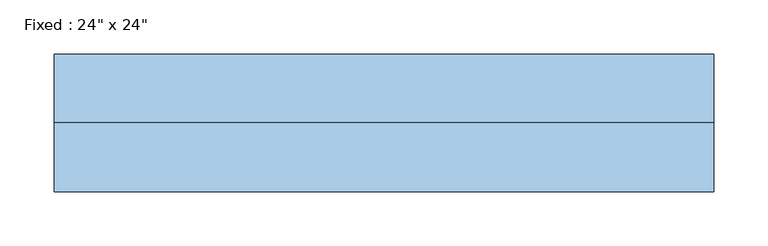
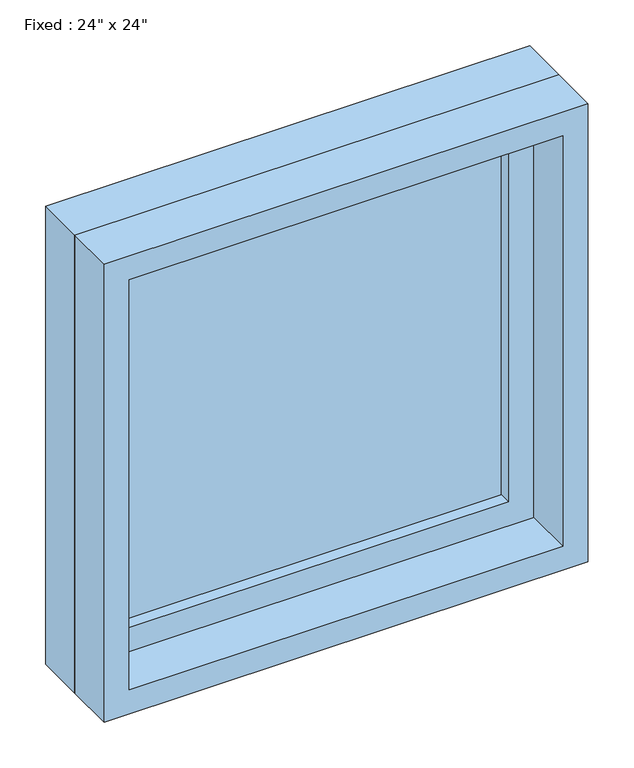
"""IFC4 building model written with IfcOpenShell, lengths in millimetres: window geometry."""

from ifc_helpers import new_model, si_unit, frame, origin, place, context, project, spatial, polyline, outline, extrude, source, transform, mapped, element, save


def window_d757e824(model_context):
    return source(origin(), model_context, "Body", "SweptSolid", [
        extrude(outline(polyline([(203.2, 15.875), (-279.4, 15.875), (-279.4, 28.575), (203.2, 28.575), (203.2, 15.875)])), frame((0.0, 0.0, 977.9), z_axis=(0.0, 0.0, 1.0), x_axis=(1.0, 0.0, 0.0)), (0.0, 0.0, 1.0), 482.6),
        extrude(outline(polyline([(1504.95, -323.85), (933.45, -323.85), (933.45, 247.65), (1504.95, 247.65), (1504.95, -323.85)]), holes=[polyline([(1460.5, -279.4), (1460.5, 203.2), (977.9, 203.2), (977.9, -279.4), (1460.5, -279.4)])]), frame((0.0, 0.0, 0.0), z_axis=(0.0, 1.0, 0.0), x_axis=(0.0, 0.0, 1.0)), (0.0, 0.0, 1.0), 44.45),
        extrude(outline(polyline([(1524.0, -342.9), (914.4, -342.9), (914.4, 266.7), (1524.0, 266.7), (1524.0, -342.9)]), holes=[polyline([(1492.25, -311.15), (1492.25, 234.95), (946.15, 234.95), (946.15, -311.15), (1492.25, -311.15)])]), frame((0.0, -63.5, 0.0), z_axis=(0.0, 1.0, 0.0), x_axis=(0.0, 0.0, 1.0)), (0.0, 0.0, 1.0), 63.5),
        extrude(outline(polyline([(1524.0, 266.7), (1524.0, -342.9), (914.4, -342.9), (914.4, 266.7), (1524.0, 266.7)]), holes=[polyline([(1504.95, 247.65), (933.45, 247.65), (933.45, -323.85), (1504.95, -323.85), (1504.95, 247.65)])]), frame((0.0, 0.0, 0.0), z_axis=(0.0, 1.0, 0.0), x_axis=(0.0, 0.0, 1.0)), (0.0, 0.0, 1.0), 63.5),
    ])


if __name__ == "__main__":
    model = new_model("IFC4")
    model_context = context("Model", 3, world=origin())
    ifc_project = project(units=[si_unit("LENGTHUNIT", "METRE", prefix="MILLI")], contexts=[model_context])
    site = spatial("IfcSite", under=ifc_project)
    building = spatial("IfcBuilding", under=site)
    placement = place(None, origin())
    window_shape = window_d757e824(model_context)
    element("IfcWindow", 1, ObjectType="Fixed : 24\" x 24\"", at=placement, inside=building, context=model_context, shape_type="MappedRepresentation", body=[
        mapped(window_shape, transform((0.0, 0.0, 0.0), x_axis=(1.0, 0.0, 0.0), y_axis=(0.0, 1.0, 0.0), z_axis=(0.0, 0.0, 1.0))),
    ])
    save(model, "model.ifc")

# Revit data of these elements
# Type "Fixed : 24\" x 24\""
#   Type Mark = "3"
#   Construction Type Id = "GSP4R"
#   Assembly Code = "B2020100"
#   Analytic Construction = "1/8 in Pilkington single glazing"
#   Visual Light Transmittance = 0.9
#   Solar Heat Gain Coefficient = 0.78
#   Heat Transfer Coefficient (U) = 0.6496 BTU/(h·ft²·°F)
#   Height = 2' - 0"
#   Default Sill Height = 3' - 0"
#   Width = 2' - 0"
#   Window Inset = 0' - 0 3/4"
#   Define Thermal Properties by = 1
#   Define Thermal Properties by = 1
#   Glass Pane Material = Glass
#   Sash Material = Sash
#   Wall Closure = (empty or 0)
# Element 1 (IfcWindow, "Fixed : 24\" x 24\"")
#   Materials on its faces: "Sash", "Glass"
# Materials
#   "Glass": class "Glass", colour RGB 0 128 192, transparency 0.75, Description = "Soda Lime Glass", Cost = 0
#   "Sash": class "Wood", colour RGB 224 178 126, transparency 0, Cost = 0
